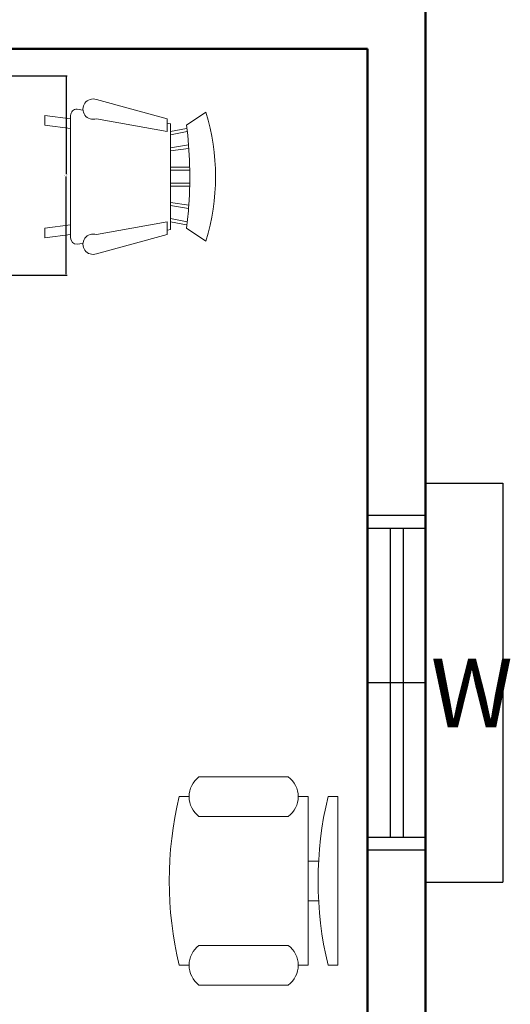
# Model space of a CAD drawing. Units: inches. Extents: x -105 to 1196, y -792 to 119.
# Tile 21 of 23: x 427 to 503, y -274 to -121. Entities that reach past the tile are written whole.
import ezdxf

# ---------------------------------------------------------------- set-up
doc = ezdxf.new("R2010")
doc.units = ezdxf.units.IN
doc.header["$MEASUREMENT"] = 0
for name, color, linetype, lineweight in [('A-ANNO-DIMS', 2, 'Continuous', 18), ('A-ANNO-TEXT', 7, 'Continuous', 25), ('A-FURN', 8, 'Continuous', 18), ('A-GLAZ', 4, 'Continuous', 25), ('A-WALL', 3, 'Continuous', 50)]:
    doc.layers.add(name, color=color, linetype=linetype, lineweight=lineweight)
doc.styles.get("Standard").update_dxf_attribs({"font": 'arial.ttf'})
doc.dimstyles.get("Standard").update_dxf_attribs({"dimtxt": 0.18, "dimasz": 0.18, "dimexe": 0.18, "dimexo": 0.0625, "dimgap": 0.09, "dimtad": 0, "dimtih": 1, "dimtoh": 1, "dimdec": 1, "dimzin": 0, "dimdsep": 46, "dimlunit": 4, "dimtxsty": 'Standard', "dimcen": 0.09, "dimadec": 0, "dimazin": 0, "dimtfac": 1, "dimtdec": 1, "dimtofl": 0, "dimtmove": 0, "dimatfit": 3, "dimfxl": 1, "dimtolj": 1, "dimtzin": 0, "dimarcsym": 0})

# ---------------------------------------------------------------- blocks, each defined once
blk = doc.blocks.new('Chair - Desk')
for p, q in [((-8.5, 0), (-8.5, -1)), ((-8.5, 0), (8.5, 0)), ((8.5, 0), (8.5, -1)), ((-2, -3), (-2, -1.9355)), ((2, -1.9576), (2, -3)), ((-8.5, -3), (-8.5, -4)), ((-8.5, -3), (8.5, -3)), ((8.5, -3), (8.5, -4)), ((-10.5, -5), (-10.5, -14)), ((-6.5, -14), (-6.5, -5)), ((6.5, -5), (6.5, -14)), ((10.5, -14), (10.5, -5)), ((-8.5, -15), (-8.5, -16)), ((8.5, -15), (8.5, -16))]:
    blk.add_line(p, q)
for centre, radius, start, end in [((0, 34.625), 36.625, 256.5803, 283.4197), ((-8.5, -6.5), 2.5, 36.8699, 143.1301), ((8.5, -6.5), 2.5, 36.8699, 143.1301), ((-8.5, -12.5), 2.5, 216.8699, 323.1301), ((8.5, -12.5), 2.5, 216.8699, 323.1301), ((0, 19.625), 36.625, 256.5803, 283.4197)]:
    blk.add_arc(centre, radius, start, end)
blk = doc.blocks.new('Chair - Rocking')
for p, q in [((-8, -4.5), (-10, -1.5)), ((8, -4.5), (10, -1.5)), ((-7.5, -4.5), (-7, -7)), ((-6.5, -7), (-7.02225, -4.43)), ((-4.5, -7), (-4.96674, -4.19951)), ((-4, -7), (-4.40532, -4.16272)), ((-1.5, -4.05012), (-1.5, -7)), ((-1, -7), (-1, -4.05012)), ((1, -7), (1, -4.04655)), ((1.5, -4.05012), (1.5, -7)), ((4, -7), (4.40187, -4.18694)), ((4.5, -7), (4.96761, -4.19437)), ((6.5, -7), (7, -4.4057)), ((7.5, -4.5), (7, -7)), ((-9, -7.5), (-12, -18.49999)), ((-7, -7.5), (-9, -7.5)), ((-9, -18.49999), (-7, -7.5)), ((-8.23428, -6.99939), (-8.3093, -7.47958)), ((-8.23041, -7), (8.23915, -7)), ((7, -7.5), (9, -7.5)), ((9, -18.49999), (7, -7.5)), ((8.31071, -7.48854), (8.23449, -7.00073)), ((9, -7.5), (12, -18.49999)), ((-10.36644, -20.64523), (-10.5, -21.49999)), ((10.5, -21.49999), (10.3575, -20.58798)), ((-9, -22.49999), (-9.5, -26.49999)), ((0, -22.49999), (-9.5, -22.49999)), ((-8, -26.49999), (-7.5, -22.49999)), ((0, -22.49999), (9.5, -22.49999)), ((8, -26.49999), (7.5, -22.49999)), ((9, -22.49999), (9.5, -26.49999)), ((-9.5, -26.49999), (-8, -26.49999)), ((9.5, -26.49999), (8, -26.49999))]:
    blk.add_line(p, q)
for centre, radius, start, end in [((0, -34.08333), 34.08333, 72.93847, 107.0615), ((0, -68.25004), 64.25, 93.92211, 97.15267), ((0, -68.25004), 64.25, 82.84733, 93.92211), ((-10.5, -18.99999), 1.58114, 161.5651, 18.43495), ((10.5, -18.99999), 1.58114, 161.5651, 18.43495), ((-9.5, -21.49999), 1, 180, 270), ((9.5, -21.49999), 1, 270, 0)]:
    blk.add_arc(centre, radius, start, end)
blk = doc.blocks.new('WIN-1200')
at = {"ltscale": 2}
for p, q in [((12, 62), (0, 62)), ((0, 0), (0, 62)), ((12, 57), (12, 62)), ((12, 5), (12, 0)), ((12, 0), (0, 0))]:
    blk.add_line(p, q, dxfattribs=at)
for p, q in [((21, 57), (12, 57)), ((21, 5), (12, 5))]:
    blk.add_line(p, q)
blk = doc.blocks.new('*D74')
at = {"layer": 'A-ANNO-DIMS', "color": 0, "lineweight": -2, "transparency": 16777216}
for p, q in [((424.99, -129.43), (434.1, -129.43)), ((433.92, -129.61), (433.92, -144.75)), ((433.92, -160.25), (433.92, -145.11)), ((424.99, -160.43), (434.1, -160.43))]:
    blk.add_line(p, q, dxfattribs=at)
at = {"layer": 'A-ANNO-DIMS', "color": 0, "transparency": 16777216}
for points in [[(433.89, -129.61), (433.95, -129.61), (433.92, -129.43)], [(433.89, -160.25), (433.95, -160.25), (433.92, -160.43)]]:
    blk.add_solid(points, dxfattribs=at)
at = {"layer": 'Defpoints', "color": 0, "transparency": 16777216}
for p in [(424.92, -129.43), (433.92, -129.43), (424.92, -160.43)]:
    blk.add_point(p, dxfattribs=at)
at = {"layer": 'A-ANNO-DIMS', "color": 0, "transparency": 16777216, "insert": (433.92, -144.93), "char_height": 0.18, "attachment_point": 5}
blk.add_mtext('\\A1;2\'-7"', dxfattribs=at)

msp = doc.modelspace()

# ---------------------------------------------------------------- linework, layer by layer
at = {"layer": 'A-GLAZ'}
for p, q in [((480.74, -199.73), (489.74, -199.73)), ((484.24, -199.73), (484.24, -247.73)), ((486.24, -199.73), (486.24, -247.73)), ((480.74, -223.73), (489.74, -223.73)), ((480.74, -247.73), (489.74, -247.73))]:
    msp.add_line(p, q, dxfattribs=at)
at = {"layer": 'A-WALL'}
for p, q in [((489.74, 69.77), (489.74, -125.23)), ((480.74, -125.23), (323.74, -125.23)), ((480.74, -125.23), (480.74, -322.23)), ((489.74, -125.23), (489.74, -508.23))]:
    msp.add_line(p, q, dxfattribs=at)

# ---------------------------------------------------------------- block references
at = {"layer": 'A-FURN', "xscale": -1, "rotation": 270}
msp.add_blockref('Chair - Rocking', (457.13, -145.12), dxfattribs=at)
at = {"layer": 'A-FURN', "xscale": 1.540628433460857, "yscale": 1.540628433460857, "zscale": 1.540628433460857, "rotation": 270}
msp.add_blockref('Chair - Desk', (476.13, -254.55), dxfattribs=at)
at = {"layer": 'A-GLAZ', "rotation": 180}
msp.add_blockref('WIN-1200', (501.74, -192.73), dxfattribs=at)

# ---------------------------------------------------------------- texts
at = {"layer": 'A-ANNO-TEXT'}
msp.add_text('W', height=10.64, dxfattribs=at).set_placement((490.54, -230.67))

# ---------------------------------------------------------------- dimensions: what is measured, and where the dimension line sits
at = {"layer": 'A-ANNO-DIMS'}
dim = msp.add_linear_dim(base=(433.92, -129.43), p1=(424.92, -160.43), p2=(424.92, -129.43), angle=90, dimstyle='Standard', override={"dimdec": 1, "dimlfac": 1, "dimrnd": 0, "dimzin": 1, "dimdsep": 46, "dimlunit": 4, "dimfrac": 2}, dxfattribs=at)
dim.commit()
dim.dimension.update_dxf_attribs({"geometry": '*D74', "text_midpoint": (433.92, -144.93)})

doc.saveas('drawing.dxf')
